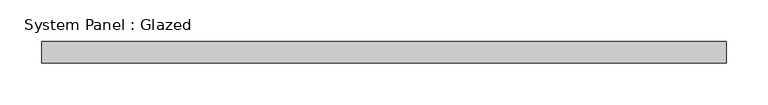
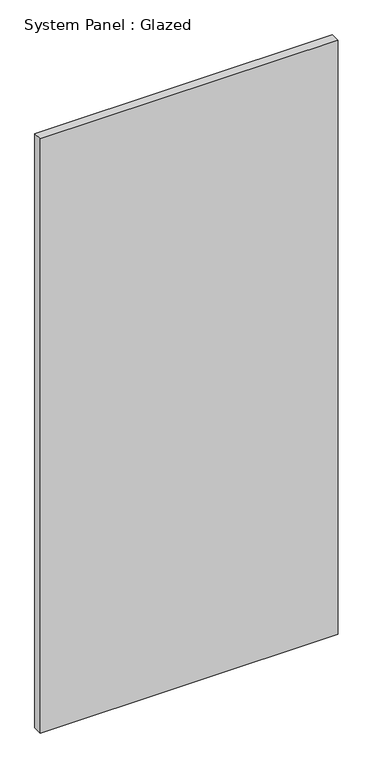
"""IFC4 building model written with IfcOpenShell, lengths in millimetres: plate geometry, System Panel : Glazed."""

from ifc_helpers import new_model, si_unit, origin, origin_with_axes, place, context, project, spatial, polyline, outline, extrude, source, transform, mapped, element, save


def system_panel_glazed_0557794d(model_context):
    return source(origin(), model_context, "Body", "SweptSolid", [
        extrude(outline(polyline([(409.575, 19.05), (-409.575, 19.05), (-409.575, 44.45), (409.575, 44.45), (409.575, 19.05)])), origin_with_axes(), (0.0, 0.0, 1.0), 1727.2),
    ])


if __name__ == "__main__":
    model = new_model("IFC4")
    model_context = context("Model", 3, world=origin())
    ifc_project = project(units=[si_unit("LENGTHUNIT", "METRE", prefix="MILLI")], contexts=[model_context])
    site = spatial("IfcSite", under=ifc_project)
    building = spatial("IfcBuilding", under=site)
    placement = place(None, origin())
    system_panel_glazed_shape = system_panel_glazed_0557794d(model_context)
    element("IfcPlate", 1, ObjectType="System Panel : Glazed", at=placement, inside=building, context=model_context, shape_type="MappedRepresentation", body=[
        mapped(system_panel_glazed_shape, transform((0.0, 0.0, 0.0), x_axis=(1.0, 0.0, 0.0), y_axis=(0.0, 1.0, 0.0), z_axis=(0.0, 0.0, 1.0))),
    ])
    save(model, "model.ifc")

# Revit data of these elements
# Type "System Panel : Glazed"
#   Construction Type Id = "GSP4R"
#   Analytic Construction = "1/8 in Pilkington single glazing"
#   Visual Light Transmittance = 0.9
#   Solar Heat Gain Coefficient = 0.86
#   Heat Transfer Coefficient (U) = 1.18115 BTU/(h·ft²·°F)
#   Define Thermal Properties by = 1
# Element 1 (IfcPlate, "System Panel : Glazed")
#   Materials on its faces: "Glass"
# Materials
#   "Glass": class "Glass", colour RGB 0 128 192, transparency 0.75, Description = "Soda Lime Glass", Cost = 0
